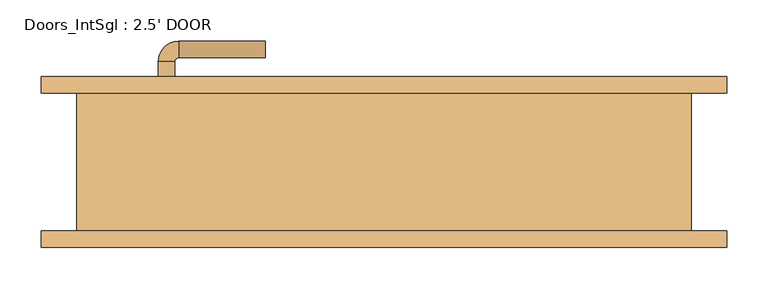
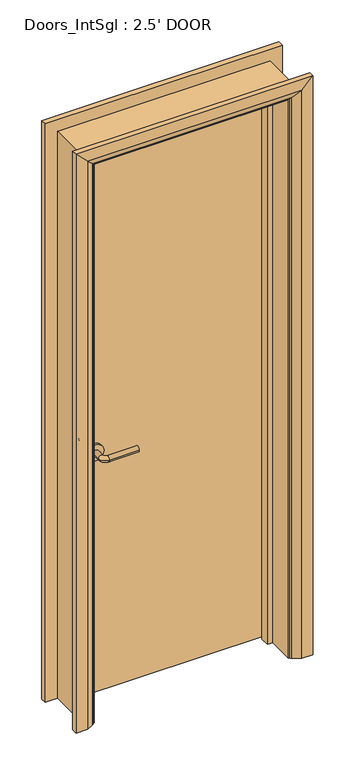
"""IFC4 building model written with IfcOpenShell, lengths in millimetres: door geometry, Doors_IntSgl : 2.5' DOOR."""

from ifc_helpers import new_model, si_unit, point, frame, frame_2d, origin, place, context, project, spatial, polyline, circle_curve, ellipse_curve, trimmed, segment, composite_curve, outline, extrude, faceted_brep, source, transform, mapped, element, save
from ifc_brep_helpers import plane_surface, cylinder_surface, revolved_surface, advanced_brep


def doors_intsgl_2_5_door_b929695a(model_context):
    return source(origin(), model_context, "Body", "SolidModel", [
        advanced_brep(
        [(-274.0, 37.82, 900.0), (-254.0, 37.82, 900.0), (-254.0, 7.82, 900.0), (-274.0, 7.82, 900.0), (-249.0, 2.82, 900.0), (-249.0, -17.18, 900.0), (-144.0, -17.18, 900.0), (-144.0, 2.82, 900.0)],
        [
            (0, 1, circle_curve(frame((-264.0, 37.82, 900.0), z_axis=(0.0, 1.0, 0.0), x_axis=(1.0, 0.0, 0.0)), 10.0)),
            (1, 0, circle_curve(frame((-264.0, 37.82, 900.0), z_axis=(0.0, 1.0, 0.0), x_axis=(1.0, 0.0, 0.0)), 10.0)),
            (1, 2),
            (2, 3, circle_curve(frame((-264.0, 7.82, 900.0), z_axis=(0.0, 1.0, 0.0), x_axis=(1.0, 0.0, 0.0)), 10.0)),
            (3, 0),
            (3, 2, circle_curve(frame((-264.0, 7.82, 900.0), z_axis=(0.0, 1.0, 0.0), x_axis=(1.0, 0.0, 0.0)), 10.0)),
            (4, 5, circle_curve(frame((-249.0, -7.18, 900.0), z_axis=(-1.0, 0.0, 0.0), x_axis=(0.0, 1.0, 0.0)), 10.0)),
            (5, 3, circle_curve(frame((-249.0, 7.82, 900.0), z_axis=(0.0, 0.0, -1.0), x_axis=(-1.0, 0.0, 0.0)), 25.0)),
            (2, 4, circle_curve(frame((-249.0, 7.82, 900.0), z_axis=(0.0, 0.0, 1.0), x_axis=(-1.0, 0.0, 0.0)), 5.0)),
            (5, 4, circle_curve(frame((-249.0, -7.18, 900.0), z_axis=(-1.0, 0.0, 0.0), x_axis=(0.0, 1.0, 0.0)), 10.0)),
            (6, 7, circle_curve(frame((-144.0, -7.18, 900.0), z_axis=(1.0, 0.0, 0.0), x_axis=(0.0, 1.0, 0.0)), 10.0)),
            (7, 6, circle_curve(frame((-144.0, -7.18, 900.0), z_axis=(1.0, 0.0, 0.0), x_axis=(0.0, 1.0, 0.0)), 10.0)),
            (4, 7),
            (6, 5),
        ],
        [
            plane_surface(frame((-264.0, 37.82, 900.0), z_axis=(0.0, 1.0, 0.0), x_axis=(0.0, 0.0, 1.0))),
            cylinder_surface(frame((-264.0, 37.82, 900.0), z_axis=(0.0, 1.0, 0.0), x_axis=(1.0, 0.0, 0.0)), 10.0),
            revolved_surface(trimmed(ellipse_curve(frame((-264.0, 7.82, 900.0), z_axis=(0.0, -1.0, 0.0), x_axis=(1.0, 0.0, 0.0)), 10.0, 10.0), [point((-274.0, 7.82, 900.0))], [point((-254.0, 7.82, 900.0))], True, "CARTESIAN"), (-249.0, 7.82, 900.0), (0.0, 0.0, -1.0)),
            revolved_surface(trimmed(ellipse_curve(frame((-264.0, 7.82, 900.0), z_axis=(0.0, -1.0, 0.0), x_axis=(1.0, 0.0, 0.0)), 10.0, 10.0), [point((-254.0, 7.82, 900.0))], [point((-274.0, 7.82, 900.0))], True, "CARTESIAN"), (-249.0, 7.82, 900.0), (0.0, 0.0, -1.0)),
            plane_surface(frame((-144.0, -7.18, 900.0), z_axis=(1.0, 0.0, 0.0), x_axis=(0.0, 0.0, 1.0))),
            cylinder_surface(frame((-249.0, -7.18, 900.0), z_axis=(-1.0, 0.0, 0.0), x_axis=(0.0, 1.0, 0.0)), 10.0),
        ],
        [
            (0, [[1, 2]]),
            (1, [[3, 4, 5, -2]]),
            (1, [[-5, 6, -3, -1]]),
            (2, [[7, 8, -4, 9]]),
            (3, [[10, -9, -6, -8]]),
            (4, [[11, 12]]),
            (5, [[13, -11, 14, -7]]),
            (5, [[-14, -12, -13, -10]]),
        ],
    ),
        extrude(outline(composite_curve([segment(trimmed(circle_curve(frame_2d((900.0, -266.5)), 30.0), [point((900.0, -296.5))], [point((900.0, -236.5))], False, "CARTESIAN"), True, "CONTINUOUS"), segment(trimmed(circle_curve(frame_2d((900.0, -266.5)), 30.0), [point((900.0, -236.5))], [point((900.0, -296.5))], False, "CARTESIAN"), True, "CONTINUOUS")], self_intersect=False)), frame((0.0, 37.82, 0.0), z_axis=(0.0, 1.0, 0.0), x_axis=(0.0, 0.0, 1.0)), (0.0, 0.0, 1.0), 8.0),
        advanced_brep(
        [(-274.0, 91.82, 900.0), (-254.0, 91.82, 900.0), (-274.0, 121.82, 900.0), (-254.0, 121.82, 900.0), (-249.0, 126.82, 900.0), (-249.0, 146.82, 900.0), (-144.0, 146.82, 900.0), (-144.0, 126.82, 900.0)],
        [
            (0, 1, circle_curve(frame((-264.0, 91.82, 900.0), z_axis=(0.0, -1.0, 0.0), x_axis=(1.0, 0.0, 0.0)), 10.0)),
            (1, 0, circle_curve(frame((-264.0, 91.82, 900.0), z_axis=(0.0, -1.0, 0.0), x_axis=(1.0, 0.0, 0.0)), 10.0)),
            (0, 2),
            (2, 3, circle_curve(frame((-264.0, 121.82, 900.0), z_axis=(0.0, -1.0, 0.0), x_axis=(1.0, 0.0, 0.0)), 10.0)),
            (3, 1),
            (3, 2, circle_curve(frame((-264.0, 121.82, 900.0), z_axis=(0.0, -1.0, 0.0), x_axis=(1.0, 0.0, 0.0)), 10.0)),
            (4, 3, circle_curve(frame((-249.0, 121.82, 900.0), z_axis=(0.0, 0.0, 1.0), x_axis=(-1.0, 0.0, 0.0)), 5.0)),
            (2, 5, circle_curve(frame((-249.0, 121.82, 900.0), z_axis=(0.0, 0.0, -1.0), x_axis=(-1.0, 0.0, 0.0)), 25.0)),
            (5, 4, circle_curve(frame((-249.0, 136.82, 900.0), z_axis=(-1.0, 0.0, 0.0), x_axis=(0.0, -1.0, 0.0)), 10.0)),
            (4, 5, circle_curve(frame((-249.0, 136.82, 900.0), z_axis=(-1.0, 0.0, 0.0), x_axis=(0.0, -1.0, 0.0)), 10.0)),
            (6, 7, circle_curve(frame((-144.0, 136.82, 900.0), z_axis=(1.0, 0.0, 0.0), x_axis=(0.0, -1.0, 0.0)), 10.0)),
            (7, 6, circle_curve(frame((-144.0, 136.82, 900.0), z_axis=(1.0, 0.0, 0.0), x_axis=(0.0, -1.0, 0.0)), 10.0)),
            (5, 6),
            (7, 4),
        ],
        [
            plane_surface(frame((-264.0, 91.82, 900.0), z_axis=(0.0, -1.0, 0.0), x_axis=(0.0, 0.0, 1.0))),
            cylinder_surface(frame((-264.0, 91.82, 900.0), z_axis=(0.0, -1.0, 0.0), x_axis=(1.0, 0.0, 0.0)), 10.0),
            revolved_surface(trimmed(ellipse_curve(frame((-264.0, 121.82, 900.0), z_axis=(0.0, -1.0, 0.0), x_axis=(1.0, 0.0, 0.0)), 10.0, 10.0), [point((-274.0, 121.82, 900.0))], [point((-254.0, 121.82, 900.0))], True, "CARTESIAN"), (-249.0, 121.82, 900.0), (0.0, 0.0, -1.0)),
            revolved_surface(trimmed(ellipse_curve(frame((-264.0, 121.82, 900.0), z_axis=(0.0, -1.0, 0.0), x_axis=(1.0, 0.0, 0.0)), 10.0, 10.0), [point((-254.0, 121.82, 900.0))], [point((-274.0, 121.82, 900.0))], True, "CARTESIAN"), (-249.0, 121.82, 900.0), (0.0, 0.0, -1.0)),
            plane_surface(frame((-144.0, 136.82, 900.0), z_axis=(1.0, 0.0, 0.0), x_axis=(0.0, 0.0, 1.0))),
            cylinder_surface(frame((-249.0, 136.82, 900.0), z_axis=(-1.0, 0.0, 0.0), x_axis=(0.0, -1.0, 0.0)), 10.0),
        ],
        [
            (0, [[1, 2]]),
            (1, [[-1, 3, 4, 5]]),
            (1, [[-2, -5, 6, -3]]),
            (2, [[7, -4, 8, 9]]),
            (3, [[-8, -6, -7, 10]]),
            (4, [[11, 12]]),
            (5, [[-9, 13, -12, 14]]),
            (5, [[-10, -14, -11, -13]]),
        ],
    ),
        extrude(outline(composite_curve([segment(trimmed(circle_curve(frame_2d((900.0, -266.5)), 30.0), [point((900.0, -296.5))], [point((900.0, -236.5))], False, "CARTESIAN"), True, "CONTINUOUS"), segment(trimmed(circle_curve(frame_2d((900.0, -266.5)), 30.0), [point((900.0, -236.5))], [point((900.0, -296.5))], False, "CARTESIAN"), True, "CONTINUOUS")], self_intersect=False)), frame((0.0, 83.82, 0.0), z_axis=(0.0, 1.0, 0.0), x_axis=(0.0, 0.0, 1.0)), (0.0, 0.0, 1.0), 8.0),
        extrude(outline(polyline([(339.0, 45.82), (-339.0, 45.82), (-339.0, 83.82), (339.0, 83.82), (339.0, 45.82)])), frame((0.0, 0.0, 8.0), z_axis=(0.0, 0.0, 1.0), x_axis=(1.0, 0.0, 0.0)), (0.0, 0.0, 1.0), 2060.0),
        advanced_brep(
        [(416.0, 103.82, 0.0), (416.0, 83.82, 0.0), (346.0, 83.82, 0.0), (350.0, 89.82, 0.0), (376.0, 103.82, 0.0), (416.0, 103.82, 2145.0), (416.0, 83.82, 2145.0), (-416.0, 83.82, 2145.0), (-416.0, 83.82, 0.0), (-346.0, 83.82, 0.0), (-346.0, 83.82, 2075.0), (346.0, 83.82, 2075.0), (350.0, 89.82, 2079.0), (376.0, 103.82, 2105.0), (-376.0, 103.82, 2105.0), (-376.0, 103.82, 0.0), (-416.0, 103.82, 0.0), (-416.0, 103.82, 2145.0), (-350.0, 89.82, 0.0), (-350.0, 89.82, 2079.0)],
        [
            (0, 1),
            (1, 2),
            (2, 3, circle_curve(frame((354.0, 82.82, 0.0), z_axis=(0.0, 0.0, -1.0), x_axis=(1.0, 0.0, 0.0)), 8.0622577)),
            (3, 4),
            (4, 0),
            (0, 5),
            (5, 6),
            (6, 1),
            (6, 7),
            (7, 8),
            (8, 9),
            (9, 10),
            (10, 11),
            (11, 2),
            (11, 12, ellipse_curve(frame((354.0, 82.82, 2083.0), z_axis=(0.7071067811865475, 0.0, -0.7071067811865475), x_axis=(-0.7071067811865474, 0.0, -0.7071067811865476)), 11.4017543, 8.0622577)),
            (12, 3),
            (12, 13),
            (13, 4),
            (13, 14),
            (14, 15),
            (15, 16),
            (16, 17),
            (17, 5),
            (7, 17),
            (16, 8),
            (15, 18),
            (18, 9, circle_curve(frame((-354.0, 82.82, 0.0), z_axis=(0.0, 0.0, -1.0), x_axis=(-1.0, 0.0, 0.0)), 8.0622577)),
            (19, 10, ellipse_curve(frame((-354.0, 82.82, 2083.0), z_axis=(-0.7071067811865475, 0.0, -0.7071067811865475), x_axis=(-0.7071067811865474, 0.0, 0.7071067811865476)), 11.4017543, 8.0622577)),
            (18, 19),
            (14, 19),
            (19, 12),
        ],
        [
            plane_surface(frame((346.0, 83.82, 0.0), z_axis=(0.0, 0.0, -1.0), x_axis=(0.0, -1.0, 0.0))),
            plane_surface(frame((416.0, 103.82, 0.0), z_axis=(1.0, 0.0, 0.0), x_axis=(0.0, 0.0, 1.0))),
            plane_surface(frame((416.0, 83.82, 0.0), z_axis=(0.0, -1.0, 0.0), x_axis=(0.0, 0.0, 1.0))),
            cylinder_surface(frame((354.0, 82.82, 0.0), z_axis=(0.0, 0.0, -1.0), x_axis=(1.0, 0.0, 0.0)), 8.0622577),
            plane_surface(frame((350.0, 89.82, 0.0), z_axis=(-0.4740998230350126, 0.880471099922178, 0.0), x_axis=(0.0, 0.0, 1.0))),
            plane_surface(frame((376.0, 103.82, 0.0), z_axis=(0.0, 1.0, 0.0), x_axis=(0.0, 0.0, 1.0))),
            plane_surface(frame((-416.0, 103.82, 2145.0), z_axis=(-1.0, 0.0, 0.0), x_axis=(0.0, 0.0, -1.0))),
            plane_surface(frame((-346.0, 83.82, 0.0), z_axis=(0.0, 0.0, -1.0), x_axis=(0.0, -1.0, 0.0))),
            cylinder_surface(frame((-354.0, 82.82, 2075.0), z_axis=(0.0, 0.0, 1.0), x_axis=(-1.0, 0.0, 0.0)), 8.0622577),
            plane_surface(frame((-350.0, 89.82, 2079.0), z_axis=(0.47409982303501824, 0.8804710999221749, 0.0), x_axis=(0.0, 0.0, -1.0))),
            plane_surface(frame((416.0, 103.82, 2145.0), z_axis=(0.0, 0.0, 1.0), x_axis=(-1.0, 0.0, 0.0))),
            cylinder_surface(frame((346.0, 82.82, 2083.0), z_axis=(1.0, 0.0, 0.0), x_axis=(0.0, 0.0, 1.0)), 8.0622577),
            plane_surface(frame((350.0, 89.82, 2079.0), z_axis=(0.0, 0.8804710999221764, -0.4740998230350154), x_axis=(-1.0, 0.0, 0.0))),
        ],
        [
            (0, [[1, 2, 3, 4, 5]]),
            (1, [[-1, 6, 7, 8]]),
            (2, [[-2, -8, 9, 10, 11, 12, 13, 14]]),
            (3, [[-3, -14, 15, 16]]),
            (4, [[-4, -16, 17, 18]]),
            (5, [[-5, -18, 19, 20, 21, 22, 23, -6]]),
            (6, [[24, -22, 25, -10]]),
            (7, [[-21, 26, 27, -11, -25]]),
            (8, [[28, -12, -27, 29]]),
            (9, [[30, -29, -26, -20]]),
            (10, [[-7, -23, -24, -9]]),
            (11, [[-15, -13, -28, 31]]),
            (12, [[-17, -31, -30, -19]]),
        ],
    ),
        extrude(outline(polyline([(0.0, -341.0), (0.0, -322.0), (2051.0, -322.0), (2051.0, 322.0), (0.0, 322.0), (0.0, 341.0), (2070.0, 341.0), (2070.0, -341.0), (0.0, -341.0)])), frame((0.0, 11.82, 0.0), z_axis=(0.0, 1.0, 0.0), x_axis=(0.0, 0.0, 1.0)), (0.0, 0.0, 1.0), 32.0),
        advanced_brep(
        [(-416.0, -103.82, 0.0), (-416.0, -83.82, 0.0), (-346.0, -83.82, 0.0), (-350.0, -89.82, 0.0), (-376.0, -103.82, 0.0), (-416.0, -103.82, 2145.0), (-416.0, -83.82, 2145.0), (-346.0, -83.82, 2075.0), (-350.0, -89.82, 2079.0), (-376.0, -103.82, 2105.0), (416.0, -103.82, 0.0), (376.0, -103.82, 0.0), (350.0, -89.82, 0.0), (346.0, -83.82, 0.0), (416.0, -83.82, 0.0), (416.0, -103.82, 2145.0), (376.0, -103.82, 2105.0), (350.0, -89.82, 2079.0), (346.0, -83.82, 2075.0), (416.0, -83.82, 2145.0)],
        [
            (0, 1),
            (1, 2),
            (2, 3, circle_curve(frame((-354.0, -82.82, 0.0), z_axis=(0.0, 0.0, -1.0), x_axis=(-1.0, 0.0, 0.0)), 8.0622577)),
            (3, 4),
            (4, 0),
            (0, 5),
            (5, 6),
            (6, 1),
            (6, 7),
            (7, 2),
            (7, 8, ellipse_curve(frame((-354.0, -82.82, 2083.0), z_axis=(-0.7071067811865475, 0.0, -0.7071067811865475), x_axis=(0.7071067811865474, 0.0, -0.7071067811865476)), 11.4017543, 8.0622577)),
            (8, 3),
            (8, 9),
            (9, 4),
            (9, 5),
            (10, 11),
            (11, 12),
            (12, 13, circle_curve(frame((354.0, -82.82, 0.0), z_axis=(0.0, 0.0, -1.0), x_axis=(1.0, 0.0, 0.0)), 8.0622577)),
            (13, 14),
            (14, 10),
            (15, 16),
            (16, 11),
            (10, 15),
            (16, 17),
            (17, 12),
            (17, 18, ellipse_curve(frame((354.0, -82.82, 2083.0), z_axis=(0.7071067811865475, 0.0, -0.7071067811865475), x_axis=(0.7071067811865474, 0.0, 0.7071067811865476)), 11.4017543, 8.0622577)),
            (18, 13),
            (18, 19),
            (19, 14),
            (19, 15),
            (5, 15),
            (19, 6),
            (18, 7),
            (17, 8),
            (16, 9),
        ],
        [
            plane_surface(frame((-346.0, -156.6210989, 0.0), z_axis=(0.0, 0.0, -1.0), x_axis=(1.0, 0.0, 0.0))),
            plane_surface(frame((-416.0, -103.82, 0.0), z_axis=(-1.0, 0.0, 0.0), x_axis=(0.0, 0.0, 1.0))),
            plane_surface(frame((-416.0, -83.82, 0.0), z_axis=(0.0, 1.0, 0.0), x_axis=(0.0, 0.0, 1.0))),
            cylinder_surface(frame((-354.0, -82.82, 0.0), z_axis=(0.0, 0.0, -1.0), x_axis=(-1.0, 0.0, 0.0)), 8.0622577),
            plane_surface(frame((-350.0, -89.82, 0.0), z_axis=(0.4740998230350183, -0.8804710999221749, 0.0), x_axis=(0.0, 0.0, 1.0))),
            plane_surface(frame((-376.0, -103.82, 0.0), z_axis=(0.0, -1.0, 0.0), x_axis=(0.0, 0.0, 1.0))),
            plane_surface(frame((346.0, -156.6210989, 0.0), z_axis=(0.0, 0.0, -1.0), x_axis=(-1.0, 0.0, 0.0))),
            plane_surface(frame((376.0, -103.82, 2105.0), z_axis=(0.0, -1.0, 0.0), x_axis=(0.0, 0.0, -1.0))),
            plane_surface(frame((350.0, -89.82, 2079.0), z_axis=(-0.4740998230350183, -0.8804710999221749, 0.0), x_axis=(0.0, 0.0, -1.0))),
            cylinder_surface(frame((354.0, -82.82, 2075.0), z_axis=(0.0, 0.0, 1.0), x_axis=(1.0, 0.0, 0.0)), 8.0622577),
            plane_surface(frame((416.0, -83.82, 2145.0), z_axis=(0.0, 1.0, 0.0), x_axis=(0.0, 0.0, -1.0))),
            plane_surface(frame((416.0, -103.82, 2145.0), z_axis=(1.0, 0.0, 0.0), x_axis=(0.0, 0.0, -1.0))),
            plane_surface(frame((-416.0, -103.82, 2145.0), z_axis=(0.0, 0.0, 1.0), x_axis=(1.0, 0.0, 0.0))),
            plane_surface(frame((-416.0, -83.82, 2145.0), z_axis=(0.0, 1.0, 0.0), x_axis=(1.0, 0.0, 0.0))),
            cylinder_surface(frame((-346.0, -82.82, 2083.0), z_axis=(-1.0, 0.0, 0.0), x_axis=(0.0, 0.0, 1.0)), 8.0622577),
            plane_surface(frame((-350.0, -89.82, 2079.0), z_axis=(0.0, -0.8804710999221749, -0.4740998230350183), x_axis=(1.0, 0.0, 0.0))),
            plane_surface(frame((-376.0, -103.82, 2105.0), z_axis=(0.0, -1.0, 0.0), x_axis=(1.0, 0.0, 0.0))),
        ],
        [
            (0, [[1, 2, 3, 4, 5]]),
            (1, [[-1, 6, 7, 8]]),
            (2, [[-2, -8, 9, 10]]),
            (3, [[-3, -10, 11, 12]]),
            (4, [[-4, -12, 13, 14]]),
            (5, [[-5, -14, 15, -6]]),
            (6, [[16, 17, 18, 19, 20]]),
            (7, [[21, 22, -16, 23]]),
            (8, [[24, 25, -17, -22]]),
            (9, [[26, 27, -18, -25]]),
            (10, [[28, 29, -19, -27]]),
            (11, [[30, -23, -20, -29]]),
            (12, [[-7, 31, -30, 32]]),
            (13, [[-9, -32, -28, 33]]),
            (14, [[-11, -33, -26, 34]]),
            (15, [[-13, -34, -24, 35]]),
            (16, [[-15, -35, -21, -31]]),
        ],
    ),
        faceted_brep([(-341.0, 83.82, 0.0), (-341.0, -83.82, 0.0), (-373.0, -83.82, 0.0), (-373.0, 83.82, 0.0), (-341.0, 83.82, 2070.0), (-341.0, -83.82, 2070.0), (-373.0, -83.82, 2102.0), (-373.0, 83.82, 2102.0), (341.0, 83.82, 0.0), (373.0, 83.82, 0.0), (373.0, -83.82, 0.0), (341.0, -83.82, 0.0), (341.0, 83.82, 2070.0), (373.0, 83.82, 2102.0), (373.0, -83.82, 2102.0), (341.0, -83.82, 2070.0)], [[[0, 1, 2, 3]], [[1, 0, 4, 5]], [[2, 1, 5, 6]], [[3, 2, 6, 7]], [[0, 3, 7, 4]], [[8, 9, 10, 11]], [[12, 13, 9, 8]], [[13, 14, 10, 9]], [[14, 15, 11, 10]], [[15, 12, 8, 11]], [[5, 4, 12, 15]], [[6, 5, 15, 14]], [[7, 6, 14, 13]], [[4, 7, 13, 12]]]),
    ])


if __name__ == "__main__":
    model = new_model("IFC4")
    model_context = context("Model", 3, world=origin())
    ifc_project = project(units=[si_unit("LENGTHUNIT", "METRE", prefix="MILLI")], contexts=[model_context])
    site = spatial("IfcSite", under=ifc_project)
    building = spatial("IfcBuilding", under=site)
    placement = place(None, origin())
    doors_intsgl_2_5_door_shape = doors_intsgl_2_5_door_b929695a(model_context)
    element("IfcDoor", 1, ObjectType="Doors_IntSgl : 2.5' DOOR", at=placement, inside=building, context=model_context, shape_type="MappedRepresentation", body=[
        mapped(doors_intsgl_2_5_door_shape, transform((0.0, 0.0, 0.0), x_axis=(1.0, 0.0, 0.0), y_axis=(0.0, 1.0, 0.0), z_axis=(0.0, 0.0, 1.0))),
    ])
    save(model, "model.ifc")

# Revit data of these elements
# Type "Doors_IntSgl : 2.5' DOOR"
#   Type Mark = "47"
#   Type Comments = "Internal Single"
#   Operation = "SingleSwingRight"
#   Manufacturer = "Revit"
#   Keynote = "L20"
#   Description = "Internal Single Door"
#   Analytic Construction = "Metal"
#   UnderCut = 0.026247 ft
#   Tolerance = 0.006562 ft
#   Thickness = 0.124672 ft
#   Thermal Resistance (R) = 0.270117 (m²·K)/W
#   Structural Tolerance = 0.026247 ft
#   StopDepth = 0.104987 ft
#   Stop Thickness = 0.062336 ft
#   Rough Width = 2.5 ft
#   Rough Height = 6.922572 ft
#   Height to Top Lock Rail = 3.28084 ft
#   Heat Transfer Coefficient (U) = 3.7021 W/(m²·K)
#   Handle Z Distance = 2.952756 ft
#   Handle X Distance = 0.246063 ft
#   Frame Thickness = 0.104987 ft
#   Door Panel Width = 2.224409 ft
#   Door Panel Thickness = 0.124672 ft
#   Door Panel Offset = 0.0 ft
#   Height = 6.922572 ft
#   Width = 2.5 ft
#   Door Panel Height = 6.75853 ft
#   Architrave Setback = 0.016404 ft
#   Vis - Ironmongery = yes
#   Material Ironmongery = Door - Handle
#   Material Frame = Door - Frame/Mullion (1)
#   Material Door = Door - Panel
#   Material Architrave = Door - Architrave
#   Visual Light Transmittance = 0
#   Solar Heat Gain Coefficient = 0
#   Function = (empty or 0)
#   Wall Closure = (empty or 0)
# Element 1 (IfcDoor, "Doors_IntSgl : 2.5' DOOR")
#   Materials on its faces: "Door - Architrave", "Door - Handle", "Door - Frame/Mullion (1)", "Door - Panel"
# Materials
#   "Door - Handle": colour RGB 0 0 0, transparency 0, Keynote = "P21", Cost = 0
#   "Door - Frame/Mullion (1)": class "Wood", colour RGB 212 179 113, transparency 0, Keynote = "L20", Cost = 0
#   "Door - Panel": class "Wood", colour RGB 210 159 95, transparency 0, Keynote = "L20", Cost = 0
#   "Door - Architrave": class "Wood", colour RGB 154 90 5, transparency 0, Keynote = "P20", Cost = 0
